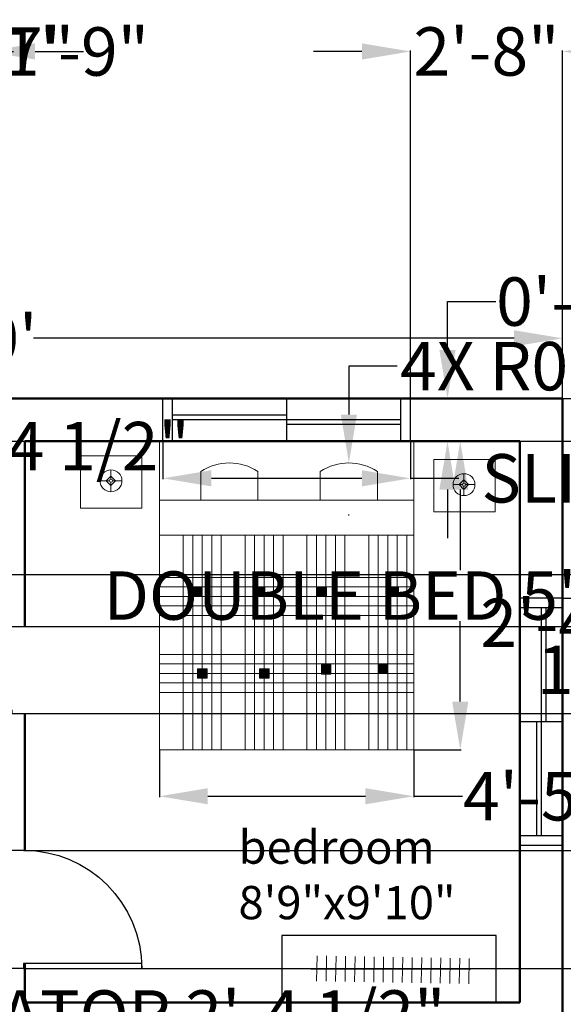
# Model space of a CAD drawing. Units: inches. Extents: x 19 to 1371, y 7 to 588.
# Tile 4 of 5: x 1092 to 1207, y 372 to 580. Entities that reach past the tile are written whole.
import ezdxf

# ---------------------------------------------------------------- set-up
doc = ezdxf.new("R2010")
doc.units = ezdxf.units.IN
doc.header["$MEASUREMENT"] = 0
for name, color, linetype, lineweight in [('A-ANNO-DIMS', 2, 'Continuous', 18), ('A-AREA-IDEN', 7, 'Continuous', 18), ('A-DOOR', 3, 'Continuous', 25), ('A-FLOR-CABN', 8, 'Continuous', 25), ('A-FURN', 8, 'Continuous', 18), ('A-FURN-PATT', 252, 'Continuous', 13), ('A-GLAZ', 4, 'Continuous', 25), ('A-WALL', 7, 'Continuous', 50)]:
    doc.layers.add(name, color=color, linetype=linetype, lineweight=lineweight)
doc.styles.get("Standard").update_dxf_attribs({"font": 'arial.ttf'})
doc.dimstyles.get("Standard").update_dxf_attribs({"dimtxt": 10.18, "dimasz": 10.18, "dimexe": 0.18, "dimexo": 0.0625, "dimgap": 0.09, "dimtad": 0, "dimtih": 1, "dimtoh": 1, "dimdec": 0, "dimzin": 0, "dimdsep": 46, "dimlunit": 3, "dimtxsty": 'Standard', "dimcen": 0.09, "dimadec": 0, "dimazin": 0, "dimtfac": 1, "dimtdec": 0, "dimtofl": 0, "dimtmove": 0, "dimatfit": 3, "dimfxl": 1, "dimtolj": 1, "dimtzin": 0, "dimarcsym": 0})

# ---------------------------------------------------------------- blocks, each defined once
blk = doc.blocks.new('*U2')
for p, q in [((0, 0), (0, -6)), ((40, 0), (40, -6))]:
    blk.add_line(p, q)
blk.add_lwpolyline([(0, 0), (0, 40), (1.75, 40), (1.75, 0)], close=True)
blk.add_arc((0, 0), 40, 0, 90)
blk = doc.blocks.new('Lamp - Table')
for p, q in [((0, 7), (0, 1)), ((-1, 0), (-7, 0)), ((0, 3), (-3, 0)), ((-3, 0), (0, -3)), ((3, 0), (0, 3)), ((0, -3), (3, 0)), ((1, 0), (7, 0)), ((0, -1), (0, -7))]:
    blk.add_line(p, q)
for radius in [7, 1]:
    blk.add_circle((0, 0), radius)
blk = doc.blocks.new('*D13')
at = {"layer": 'A-ANNO-DIMS', "color": 0, "lineweight": -2, "transparency": 16777216}
for p, q in [((966.44, 499.95), (966.44, 512.71)), ((976.62, 512.53), (1077.63, 512.53)), ((1196.26, 512.53), (1095.26, 512.53)), ((1206.44, 499.95), (1206.44, 512.71))]:
    blk.add_line(p, q, dxfattribs=at)
at = {"layer": 'A-ANNO-DIMS', "color": 0, "transparency": 16777216}
for points in [[(976.62, 514.22), (976.62, 510.83), (966.44, 512.53)], [(1196.26, 514.22), (1196.26, 510.83), (1206.44, 512.53)]]:
    blk.add_solid(points, dxfattribs=at)
at = {"layer": 'Defpoints', "color": 0, "transparency": 16777216}
for p in [(1206.44, 512.53), (966.44, 499.89), (1206.44, 499.89)]:
    blk.add_point(p, dxfattribs=at)
at = {"layer": 'A-ANNO-DIMS', "color": 0, "transparency": 16777216, "insert": (1086.44, 512.53), "char_height": 10.18, "attachment_point": 5}
blk.add_mtext("\\A1;20'", dxfattribs=at)
blk = doc.blocks.new('BED-DOUBLE-PLAN')
h = blk.add_hatch(color=256)
h.dxf.hatch_style = 1
h.paths.add_polyline_path([(9, 34.29), (7, 34.29), (7, 32.29), (9, 32.29)])
h = blk.add_hatch(color=256)
h.dxf.hatch_style = 1
h.paths.add_polyline_path([(22.14, 34.29), (20.14, 34.29), (20.14, 32.29), (22.14, 32.29)])
h = blk.add_hatch(color=256)
h.dxf.hatch_style = 1
h.paths.add_polyline_path([(35.09, 34.29), (33.09, 34.29), (33.09, 32.29), (35.09, 32.29)])
h = blk.add_hatch(color=256)
h.dxf.hatch_style = 1
h.paths.add_polyline_path([(50.26, 34.29), (48.26, 34.29), (48.26, 32.29), (50.26, 32.29)])
h = blk.add_hatch(color=256)
h.dxf.hatch_style = 1
h.paths.add_polyline_path([(10.04, 17.06), (8.04, 17.06), (8.04, 15.06), (10.04, 15.06)])
h = blk.add_hatch(color=256)
h.dxf.hatch_style = 1
h.paths.add_polyline_path([(23.04, 17.06), (21.04, 17.06), (21.04, 15.06), (23.04, 15.06)])
h = blk.add_hatch(color=256)
h.dxf.hatch_style = 1
h.paths.add_polyline_path([(36.04, 17.94), (34.04, 17.94), (34.04, 15.94), (36.04, 15.94)])
h = blk.add_hatch(color=256)
h.dxf.hatch_style = 1
h.paths.add_polyline_path([(47.99, 18.12), (45.99, 18.12), (45.99, 16.12), (47.99, 16.12)])
for p, q in [((8.7, 52.54), (8.7, 58.53)), ((20.7, 52.54), (20.7, 58.53)), ((33.82, 52.54), (33.82, 58.53)), ((45.82, 52.54), (45.82, 58.53)), ((53.49, 52.54), (0, 52.54)), ((0, 45.16), (53.49, 45.16)), ((0, 45.16), (5, 45.16)), ((5, 45.16), (5, 0)), ((7, 45.16), (7, 0)), ((9, 45.16), (9, 0)), ((11, 45.16), (11, 0)), ((13, 45.16), (13, 0)), ((18, 45.16), (18, 0)), ((20, 45.16), (20, 0)), ((22, 45.16), (22, 0)), ((24, 45.16), (24, 0)), ((26, 45.16), (26, 0)), ((31, 45.16), (31, 0)), ((33, 45.16), (33, 0)), ((35, 45.16), (35, 0)), ((37, 45.16), (37, 0)), ((39, 45.16), (39, 0)), ((44, 45.16), (44, 0)), ((46, 45.16), (46, 0)), ((48, 45.16), (48, 0)), ((50, 45.16), (50, 0)), ((52, 45.16), (52, 0)), ((0, 36.29), (53.49, 36.29)), ((0, 34.29), (53.49, 34.29)), ((0, 32.29), (53.49, 32.29)), ((0, 30.29), (53.49, 30.29)), ((0, 28.29), (53.49, 28.29)), ((0, 20.08), (53.49, 20.08)), ((0, 18.08), (53.49, 18.08)), ((0, 16.08), (53.49, 16.08)), ((0, 14.08), (53.49, 14.08)), ((0, 12.08), (53.49, 12.08)), ((5, 0), (5, 4.72)), ((5, 4.72), (5, 0))]:
    blk.add_line(p, q)
for points in [[(53.49, 64.91), (0, 64.91), (0, 0), (53.49, 0)], [(7, 34.29), (9, 34.29), (9, 32.29), (7, 32.29)], [(20.14, 34.29), (22.14, 34.29), (22.14, 32.29), (20.14, 32.29)], [(33.09, 34.29), (35.09, 34.29), (35.09, 32.29), (33.09, 32.29)], [(48.26, 34.29), (50.26, 34.29), (50.26, 32.29), (48.26, 32.29)], [(8.04, 17.06), (10.04, 17.06), (10.04, 15.06), (8.04, 15.06)], [(21.04, 17.06), (23.04, 17.06), (23.04, 15.06), (21.04, 15.06)], [(34.04, 17.94), (36.04, 17.94), (36.04, 15.94), (34.04, 15.94)], [(45.99, 18.12), (47.99, 18.12), (47.99, 16.12), (45.99, 16.12)]]:
    blk.add_lwpolyline(points, close=True)
for centre in [(14.7, 49.44), (39.82, 49.44)]:
    blk.add_arc(centre, 10.9, 56.5918, 123.4082)
blk = doc.blocks.new('WIN-SLIDING-48')
for p, q in [((0, 0), (0, 9)), ((2, 0), (2, 9)), ((26, 0), (26, 9)), ((50, 0), (50, 9)), ((52, 0), (52, 9)), ((26, 5.5), (2, 5.5)), ((50, 4.5), (2, 4.5)), ((50, 3.5), (26, 3.5))]:
    blk.add_line(p, q)
blk = doc.blocks.new('TABLE-BEDSIDE')
blk.add_lwpolyline([(0, 11.01), (12.94, 11.01), (12.94, 0), (0, 0)], close=True)
blk = doc.blocks.new('*D20')
at = {"layer": 'A-ANNO-DIMS', "color": 0, "lineweight": -2, "transparency": 16777216}
for p, q in [((1175.27, 490.89), (1185.12, 490.89)), ((1184.94, 480.71), (1184.94, 463.79)), ((1184.94, 436.16), (1184.94, 453.08)), ((1175.27, 425.98), (1185.12, 425.98))]:
    blk.add_line(p, q, dxfattribs=at)
at = {"layer": 'A-ANNO-DIMS', "color": 0, "transparency": 16777216}
for points in [[(1183.24, 480.71), (1186.64, 480.71), (1184.94, 490.89)], [(1183.24, 436.16), (1186.64, 436.16), (1184.94, 425.98)]]:
    blk.add_solid(points, dxfattribs=at)
at = {"layer": 'Defpoints', "color": 0, "transparency": 16777216}
for p in [(1175.2, 490.89), (1184.94, 490.89), (1175.2, 425.98)]:
    blk.add_point(p, dxfattribs=at)
at = {"layer": 'A-ANNO-DIMS', "color": 0, "transparency": 16777216, "insert": (1184.94, 458.44), "char_height": 10.18, "attachment_point": 5}
blk.add_mtext('\\A1;DOUBLE BED 5\'-5" TYP.', dxfattribs=at)
blk = doc.blocks.new('*D21')
at = {"layer": 'A-ANNO-DIMS', "color": 0, "lineweight": -2, "transparency": 16777216}
for p, q in [((1121.71, 425.92), (1121.71, 416.06)), ((1175.2, 425.92), (1175.2, 416.06)), ((1131.89, 416.24), (1165.02, 416.24)), ((1175.2, 416.24), (1185.38, 416.24))]:
    blk.add_line(p, q, dxfattribs=at)
at = {"layer": 'A-ANNO-DIMS', "color": 0, "transparency": 16777216}
for points in [[(1131.89, 417.94), (1131.89, 414.55), (1121.71, 416.24)], [(1165.02, 417.94), (1165.02, 414.55), (1175.2, 416.24)]]:
    blk.add_solid(points, dxfattribs=at)
at = {"layer": 'Defpoints', "color": 0, "transparency": 16777216}
for p in [(1121.71, 425.98), (1175.2, 425.98), (1175.2, 416.24)]:
    blk.add_point(p, dxfattribs=at)
at = {"layer": 'A-ANNO-DIMS', "color": 0, "transparency": 16777216, "insert": (1228.56, 416.24), "char_height": 10.18, "attachment_point": 5}
blk.add_mtext('\\A1;4\'-5 1/2" TYP.', dxfattribs=at)
blk = doc.blocks.new('*D30')
at = {"layer": 'A-ANNO-DIMS', "color": 0, "lineweight": -2, "transparency": 16777216}
for p, q in [((1122.46, 490.83), (1122.46, 482.91)), ((1174.46, 490.83), (1174.46, 482.91)), ((1132.64, 483.09), (1164.28, 483.09)), ((1174.46, 483.09), (1184.64, 483.09))]:
    blk.add_line(p, q, dxfattribs=at)
at = {"layer": 'A-ANNO-DIMS', "color": 0, "transparency": 16777216}
for points in [[(1132.64, 484.79), (1132.64, 481.39), (1122.46, 483.09)], [(1164.28, 484.79), (1164.28, 481.39), (1174.46, 483.09)]]:
    blk.add_solid(points, dxfattribs=at)
at = {"layer": 'Defpoints', "color": 0, "transparency": 16777216}
for p in [(1122.46, 490.89), (1174.46, 490.89), (1174.46, 483.09)]:
    blk.add_point(p, dxfattribs=at)
at = {"layer": 'A-ANNO-DIMS', "color": 0, "transparency": 16777216, "insert": (1279.33, 483.09), "char_height": 10.18, "attachment_point": 5}
blk.add_mtext('\\A1;SLIDING WINDOW 4\'-4" TYP.', dxfattribs=at)
blk = doc.blocks.new('*D31')
at = {"layer": 'A-ANNO-DIMS', "color": 0, "lineweight": -2, "transparency": 16777216}
for p, q in [((1182.26, 510.07), (1182.26, 520.25)), ((1182.26, 520.25), (1192.44, 520.25)), ((1174.52, 499.89), (1182.44, 499.89)), ((1174.52, 490.89), (1182.44, 490.89)), ((1182.26, 480.71), (1182.26, 470.53))]:
    blk.add_line(p, q, dxfattribs=at)
at = {"layer": 'A-ANNO-DIMS', "color": 0, "transparency": 16777216}
for points in [[(1180.56, 510.07), (1183.95, 510.07), (1182.26, 499.89)], [(1180.56, 480.71), (1183.95, 480.71), (1182.26, 490.89)]]:
    blk.add_solid(points, dxfattribs=at)
at = {"layer": 'Defpoints', "color": 0, "transparency": 16777216}
for p in [(1174.46, 499.89), (1182.26, 499.89), (1174.46, 490.89)]:
    blk.add_point(p, dxfattribs=at)
at = {"layer": 'A-ANNO-DIMS', "color": 0, "transparency": 16777216, "insert": (1223.55, 520.25), "char_height": 10.18, "attachment_point": 5}
blk.add_mtext('\\A1;0\'-9" TYP.', dxfattribs=at)
blk = doc.blocks.new('*D32')
at = {"layer": 'A-ANNO-DIMS', "color": 0, "lineweight": -2, "transparency": 16777216}
for p, q in [((992.39, 489.86), (982.21, 489.86)), ((1002.57, 487.44), (1002.57, 490.04)), ((1019.13, 487.44), (1019.13, 490.04)), ((1029.31, 489.86), (1039.49, 489.86))]:
    blk.add_line(p, q, dxfattribs=at)
at = {"layer": 'A-ANNO-DIMS', "color": 0, "transparency": 16777216}
for points in [[(992.39, 491.56), (992.39, 488.17), (1002.57, 489.86)], [(1029.31, 491.56), (1029.31, 488.17), (1019.13, 489.86)]]:
    blk.add_solid(points, dxfattribs=at)
at = {"layer": 'Defpoints', "color": 0, "transparency": 16777216}
for p in [(1019.13, 489.86), (1002.57, 487.38), (1019.13, 487.38)]:
    blk.add_point(p, dxfattribs=at)
at = {"layer": 'A-ANNO-DIMS', "color": 0, "transparency": 16777216, "insert": (1083.52, 489.86), "char_height": 10.18, "attachment_point": 5}
blk.add_mtext('\\A1;SINK 1\'-4 1/2"', dxfattribs=at)
blk = doc.blocks.new('*D36')
at = {"layer": 'A-ANNO-DIMS', "color": 0, "lineweight": -2, "transparency": 16777216}
for p, q in [((980.44, 374.59), (980.44, 370.17)), ((1009.08, 374.59), (1009.08, 370.17)), ((990.62, 370.35), (998.9, 370.35)), ((1009.08, 370.35), (1019.26, 370.35))]:
    blk.add_line(p, q, dxfattribs=at)
at = {"layer": 'A-ANNO-DIMS', "color": 0, "transparency": 16777216}
for points in [[(990.62, 372.05), (990.62, 368.66), (980.44, 370.35)], [(998.9, 372.05), (998.9, 368.66), (1009.08, 370.35)]]:
    blk.add_solid(points, dxfattribs=at)
at = {"layer": 'Defpoints', "color": 0, "transparency": 16777216}
for p in [(980.44, 374.65), (1009.08, 374.65), (1009.08, 370.35)]:
    blk.add_point(p, dxfattribs=at)
at = {"layer": 'A-ANNO-DIMS', "color": 0, "transparency": 16777216, "insert": (1102.94, 370.35), "char_height": 10.18, "attachment_point": 5}
blk.add_mtext('\\A1;REFRIGERATOR 2\'-4 1/2"', dxfattribs=at)
blk = doc.blocks.new('*D46')
at = {"layer": 'A-ANNO-DIMS', "color": 0, "lineweight": -2, "transparency": 16777216}
for p, q in [((1035.21, 572.84), (1025.03, 572.84)), ((1045.39, 211.95), (1045.39, 573.02)), ((1085.39, 211.95), (1085.39, 573.02)), ((1095.57, 572.84), (1105.75, 572.84))]:
    blk.add_line(p, q, dxfattribs=at)
at = {"layer": 'A-ANNO-DIMS', "color": 0, "transparency": 16777216}
for points in [[(1035.21, 574.54), (1035.21, 571.14), (1045.39, 572.84)], [(1095.57, 574.54), (1095.57, 571.14), (1085.39, 572.84)]]:
    blk.add_solid(points, dxfattribs=at)
at = {"layer": 'Defpoints', "color": 0, "transparency": 16777216}
for p in [(1085.39, 572.84), (1045.39, 211.89), (1085.39, 211.89)]:
    blk.add_point(p, dxfattribs=at)
at = {"layer": 'A-ANNO-DIMS', "color": 0, "transparency": 16777216, "insert": (1065.39, 572.84), "char_height": 10.18, "attachment_point": 5}
blk.add_mtext('\\A1;3\'-4"', dxfattribs=at)
blk = doc.blocks.new('*D48')
at = {"layer": 'A-ANNO-DIMS', "color": 0, "lineweight": -2, "transparency": 16777216}
for p, q in [((1228.39, 404.87), (1228.39, 415.05)), ((1228.39, 415.05), (1238.57, 415.05)), ((1093.5, 404.87), (1228.57, 404.87)), ((1228.39, 390.2), (1228.39, 394.69)), ((1093.23, 380.02), (1228.57, 380.02))]:
    blk.add_line(p, q, dxfattribs=at)
at = {"layer": 'A-ANNO-DIMS', "color": 0, "transparency": 16777216}
for points in [[(1226.7, 394.69), (1230.09, 394.69), (1228.39, 404.87)], [(1226.7, 390.2), (1230.09, 390.2), (1228.39, 380.02)]]:
    blk.add_solid(points, dxfattribs=at)
at = {"layer": 'Defpoints', "color": 0, "transparency": 16777216}
for p in [(1093.44, 404.87), (1228.39, 404.87), (1093.17, 380.02)]:
    blk.add_point(p, dxfattribs=at)
at = {"layer": 'A-ANNO-DIMS', "color": 0, "transparency": 16777216, "insert": (1252.28, 415.05), "char_height": 10.18, "attachment_point": 5}
blk.add_mtext('\\A1;2\'-1"', dxfattribs=at)
blk = doc.blocks.new('*D50')
at = {"layer": 'A-ANNO-DIMS', "color": 0, "lineweight": -2, "transparency": 16777216}
for p, q in [((1228.39, 462.14), (1228.39, 472.32)), ((1093.5, 451.96), (1228.57, 451.96)), ((1093.5, 433.64), (1228.57, 433.64)), ((1228.39, 423.46), (1228.39, 413.28))]:
    blk.add_line(p, q, dxfattribs=at)
at = {"layer": 'A-ANNO-DIMS', "color": 0, "transparency": 16777216}
for points in [[(1226.7, 462.14), (1230.09, 462.14), (1228.39, 451.96)], [(1226.7, 423.46), (1230.09, 423.46), (1228.39, 433.64)]]:
    blk.add_solid(points, dxfattribs=at)
at = {"layer": 'Defpoints', "color": 0, "transparency": 16777216}
for p in [(1093.44, 451.96), (1228.39, 451.96), (1093.44, 433.64)]:
    blk.add_point(p, dxfattribs=at)
at = {"layer": 'A-ANNO-DIMS', "color": 0, "transparency": 16777216, "insert": (1228.39, 442.8), "char_height": 10.18, "attachment_point": 5}
blk.add_mtext('\\A1;1\'-6 1/2"', dxfattribs=at)
blk = doc.blocks.new('*D61')
at = {"layer": 'A-ANNO-DIMS', "color": 0, "lineweight": -2, "transparency": 16777216}
for p, q in [((1206.5, 499.89), (1228.57, 499.89)), ((1228.39, 489.71), (1228.39, 484.18)), ((1228.39, 468.07), (1228.39, 473.6)), ((1206.5, 457.89), (1228.57, 457.89))]:
    blk.add_line(p, q, dxfattribs=at)
at = {"layer": 'A-ANNO-DIMS', "color": 0, "transparency": 16777216}
for points in [[(1226.7, 489.71), (1230.09, 489.71), (1228.39, 499.89)], [(1226.7, 468.07), (1230.09, 468.07), (1228.39, 457.89)]]:
    blk.add_solid(points, dxfattribs=at)
at = {"layer": 'Defpoints', "color": 0, "transparency": 16777216}
for p in [(1206.44, 499.89), (1206.44, 457.89), (1228.39, 457.89)]:
    blk.add_point(p, dxfattribs=at)
at = {"layer": 'A-ANNO-DIMS', "color": 0, "transparency": 16777216, "insert": (1228.39, 478.89), "char_height": 10.18, "attachment_point": 5}
blk.add_mtext('\\A1;3\'-6"', dxfattribs=at)
blk = doc.blocks.new('*D62')
at = {"layer": 'A-ANNO-DIMS', "color": 0, "lineweight": -2, "transparency": 16777216}
for p, q in [((1228.39, 377.07), (1228.39, 387.25)), ((1197.5, 366.89), (1228.57, 366.89)), ((1197.5, 359.89), (1228.57, 359.89)), ((1228.39, 349.71), (1228.39, 339.53)), ((1228.39, 339.53), (1218.21, 339.53))]:
    blk.add_line(p, q, dxfattribs=at)
at = {"layer": 'A-ANNO-DIMS', "color": 0, "transparency": 16777216}
for points in [[(1226.7, 377.07), (1230.09, 377.07), (1228.39, 366.89)], [(1226.7, 349.71), (1230.09, 349.71), (1228.39, 359.89)]]:
    blk.add_solid(points, dxfattribs=at)
at = {"layer": 'Defpoints', "color": 0, "transparency": 16777216}
for p in [(1197.44, 366.89), (1197.44, 359.89), (1228.39, 359.89)]:
    blk.add_point(p, dxfattribs=at)
at = {"layer": 'A-ANNO-DIMS', "color": 0, "transparency": 16777216, "insert": (1204.59, 339.53), "char_height": 10.18, "attachment_point": 5}
blk.add_mtext('\\A1;0\'-7"', dxfattribs=at)
blk = doc.blocks.new('*D64')
at = {"layer": 'A-ANNO-DIMS', "color": 0, "lineweight": -2, "transparency": 16777216}
for p, q in [((1037.26, 572.84), (1027.08, 572.84)), ((1047.44, 490.95), (1047.44, 573.02)), ((1054.44, 490.95), (1054.44, 573.02)), ((1064.62, 572.84), (1074.8, 572.84))]:
    blk.add_line(p, q, dxfattribs=at)
at = {"layer": 'A-ANNO-DIMS', "color": 0, "transparency": 16777216}
for points in [[(1037.26, 574.54), (1037.26, 571.14), (1047.44, 572.84)], [(1064.62, 574.54), (1064.62, 571.14), (1054.44, 572.84)]]:
    blk.add_solid(points, dxfattribs=at)
at = {"layer": 'Defpoints', "color": 0, "transparency": 16777216}
for p in [(1054.44, 572.84), (1047.44, 490.89), (1054.44, 490.89)]:
    blk.add_point(p, dxfattribs=at)
at = {"layer": 'A-ANNO-DIMS', "color": 0, "transparency": 16777216, "insert": (1088.42, 572.84), "char_height": 10.18, "attachment_point": 5}
blk.add_mtext('\\A1;0\'-7"', dxfattribs=at)
blk = doc.blocks.new('*D65')
at = {"layer": 'A-ANNO-DIMS', "color": 0, "lineweight": -2, "transparency": 16777216}
for p, q in [((1164.28, 572.84), (1154.1, 572.84)), ((1174.46, 499.95), (1174.46, 573.02)), ((1206.44, 499.95), (1206.44, 573.02)), ((1216.62, 572.84), (1226.8, 572.84))]:
    blk.add_line(p, q, dxfattribs=at)
at = {"layer": 'A-ANNO-DIMS', "color": 0, "transparency": 16777216}
for points in [[(1164.28, 574.54), (1164.28, 571.14), (1174.46, 572.84)], [(1216.62, 574.54), (1216.62, 571.14), (1206.44, 572.84)]]:
    blk.add_solid(points, dxfattribs=at)
at = {"layer": 'Defpoints', "color": 0, "transparency": 16777216}
for p in [(1206.44, 572.84), (1174.46, 499.89), (1206.44, 499.89)]:
    blk.add_point(p, dxfattribs=at)
at = {"layer": 'A-ANNO-DIMS', "color": 0, "transparency": 16777216, "insert": (1190.45, 572.84), "char_height": 10.18, "attachment_point": 5}
blk.add_mtext('\\A1;2\'-8"', dxfattribs=at)
blk = doc.blocks.new('*D68')
at = {"layer": 'A-ANNO-DIMS', "color": 0, "lineweight": -2, "transparency": 16777216}
for p, q in [((1059.87, 490.95), (1059.87, 573.02)), ((1070.05, 572.84), (1070.69, 572.84)), ((1080.87, 490.95), (1080.87, 573.02)), ((1080.87, 572.84), (1091.05, 572.84))]:
    blk.add_line(p, q, dxfattribs=at)
at = {"layer": 'A-ANNO-DIMS', "color": 0, "transparency": 16777216}
for points in [[(1070.05, 574.54), (1070.05, 571.14), (1059.87, 572.84)], [(1070.69, 574.54), (1070.69, 571.14), (1080.87, 572.84)]]:
    blk.add_solid(points, dxfattribs=at)
at = {"layer": 'Defpoints', "color": 0, "transparency": 16777216}
for p in [(1080.87, 572.84), (1059.87, 490.89), (1080.87, 490.89)]:
    blk.add_point(p, dxfattribs=at)
at = {"layer": 'A-ANNO-DIMS', "color": 0, "transparency": 16777216, "insert": (1104.19, 572.84), "char_height": 10.18, "attachment_point": 5}
blk.add_mtext('\\A1;1\'-9"', dxfattribs=at)
blk = doc.blocks.new('*D69')
at = {"layer": 'A-ANNO-DIMS', "color": 0, "lineweight": -2, "transparency": 16777216}
for p, q in [((1080.93, 490.89), (1228.57, 490.89)), ((1228.39, 480.71), (1228.39, 473.07)), ((1070.43, 462.89), (1228.57, 462.89)), ((1228.39, 462.89), (1228.39, 452.71)), ((1228.39, 452.71), (1218.21, 452.71))]:
    blk.add_line(p, q, dxfattribs=at)
at = {"layer": 'A-ANNO-DIMS', "color": 0, "transparency": 16777216}
for points in [[(1226.7, 480.71), (1230.09, 480.71), (1228.39, 490.89)], [(1226.7, 473.07), (1230.09, 473.07), (1228.39, 462.89)]]:
    blk.add_solid(points, dxfattribs=at)
at = {"layer": 'Defpoints', "color": 0, "transparency": 16777216}
for p in [(1080.87, 490.89), (1070.37, 462.89), (1228.39, 462.89)]:
    blk.add_point(p, dxfattribs=at)
at = {"layer": 'A-ANNO-DIMS', "color": 0, "transparency": 16777216, "insert": (1204.51, 452.71), "char_height": 10.18, "attachment_point": 5}
blk.add_mtext('\\A1;2\'-4"', dxfattribs=at)
blk = doc.blocks.new('*D75')
at = {"layer": 'A-ANNO-DIMS', "color": 0, "lineweight": -2, "transparency": 16777216}
for p, q in [((1171.71, 506.67), (1161.53, 506.67)), ((1161.53, 506.67), (1161.53, 496.49)), ((1161.44, 475.42), (1161.62, 475.42)), ((1161.53, 475.33), (1161.53, 475.51))]:
    blk.add_line(p, q, dxfattribs=at)
at = {"layer": 'A-ANNO-DIMS', "color": 0, "transparency": 16777216}
blk.add_solid([(1159.84, 496.49), (1163.23, 496.49), (1161.53, 486.31)], dxfattribs=at)
at = {"layer": 'Defpoints', "color": 0, "transparency": 16777216}
for p in [(1161.53, 486.31), (1161.53, 475.42)]:
    blk.add_point(p, dxfattribs=at)
at = {"layer": 'A-ANNO-DIMS', "color": 0, "transparency": 16777216, "insert": (1205.3, 506.67), "char_height": 10.18, "attachment_point": 5}
blk.add_mtext('\\A1;4X R0\'-11"', dxfattribs=at)

msp = doc.modelspace()

# ---------------------------------------------------------------- hatches: boundary and pattern name
at = {"layer": 'A-FURN-PATT'}
h = msp.add_hatch(dxfattribs=at)
h.set_pattern_fill('ANSI31', color=256, scale=15.99746, angle=43.9757, style=0)
h.paths.add_polyline_path([(1154.7, 377.38), (1186.79, 376.81), (1186.89, 382.15), (1154.79, 382.72)])

# ---------------------------------------------------------------- linework, layer by layer
at = {"layer": 'A-FLOR-CABN'}
for p, q in [((1192.51, 386.93), (1147.46, 386.93)), ((1147.46, 386.93), (1147.46, 372.89)), ((1192.51, 372.89), (1192.51, 386.93)), ((1153.52, 379.99), (1187.16, 379.99))]:
    msp.add_line(p, q, dxfattribs=at)
at = {"layer": 'A-WALL'}
for p, q in [((966.44, 499.89), (1206.44, 499.89)), ((1206.44, 499.89), (1206.44, 139.89)), ((1093.44, 490.89), (1197.44, 490.89)), ((1093.44, 451.96), (1093.44, 490.89)), ((1197.44, 490.89), (1197.44, 372.89)), ((1093.44, 404.87), (1093.44, 433.64)), ((1093.44, 372.89), (1093.44, 381.11)), ((1093.44, 372.89), (1197.44, 372.89))]:
    msp.add_line(p, q, dxfattribs=at)

# ---------------------------------------------------------------- block references
at = {"layer": 'A-DOOR'}
for p, xscale, yscale, zscale, rotation in [((1090.69, 433.64), 0.4579245056729436, 0.4579245056729436, 0.4579245056729436, 90), ((1093.17, 380.02), -0.6212879094378088, 0.6212879094378088, 0.6212879094378088, 270)]:
    msp.add_blockref('*U2', p, dxfattribs=dict(at, xscale=xscale, yscale=yscale, zscale=zscale, rotation=rotation))
at = {"layer": 'A-FURN'}
for name, p in [('BED-DOUBLE-PLAN', (1121.71, 425.98)), ('TABLE-BEDSIDE', (1105.11, 476.84)), ('TABLE-BEDSIDE', (1179.36, 476.05))]:
    msp.add_blockref(name, p, dxfattribs=at)
at = {"layer": 'A-FURN', "xscale": 0.3285708312946518, "yscale": 0.3285708312946518, "zscale": 0.3285708312946518}
for p in [(1111.53, 482.58), (1185.72, 481.76)]:
    msp.add_blockref('Lamp - Table', p, dxfattribs=at)
at = {"layer": 'A-GLAZ'}
msp.add_blockref('WIN-SLIDING-48', (1122.46, 490.89), dxfattribs=at)
at = {"layer": 'A-GLAZ', "rotation": 90.00000000000011}
msp.add_blockref('WIN-SLIDING-48', (1206.44, 405.89), dxfattribs=at)

# ---------------------------------------------------------------- texts
at = {"layer": 'A-AREA-IDEN', "insert": (1138.33, 409.05), "char_height": 7, "attachment_point": 1}
msp.add_mtext_dynamic_manual_height_columns('bedroom\\P8\'9"x9\'10"', width=53.7683, gutter_width=1, heights=[0], dxfattribs=at)

# ---------------------------------------------------------------- dimensions: what is measured, and where the dimension line sits
at = {"layer": 'A-ANNO-DIMS'}
for base, p1, p2, override, picture, middle in [((1085.39, 572.84), (1045.39, 211.89), (1085.39, 211.89), {"dimdec": 1, "dimlfac": 1, "dimrnd": 0, "dimzin": 1, "dimdsep": 46, "dimlunit": 4, "dimfrac": 2}, '*D46', (1065.39, 572.84)), ((1054.44, 572.84), (1047.44, 490.89), (1054.44, 490.89), {"dimdec": 1, "dimlfac": 1, "dimrnd": 0, "dimzin": 1, "dimdsep": 46, "dimlunit": 4, "dimfrac": 2}, '*D64', (1088.42, 572.84)), ((1080.87, 572.84), (1059.87, 490.89), (1080.87, 490.89), {"dimdec": 1, "dimlfac": 1, "dimrnd": 0, "dimzin": 1, "dimdsep": 46, "dimlunit": 4, "dimfrac": 2}, '*D68', (1104.19, 572.84)), ((1206.44, 572.84), (1174.46, 499.89), (1206.44, 499.89), {"dimdec": 1, "dimlfac": 1, "dimrnd": 0, "dimzin": 1, "dimdsep": 46, "dimlunit": 4, "dimfrac": 2}, '*D65', (1190.45, 572.84)), ((1206.44, 512.53), (966.44, 499.89), (1206.44, 499.89), {"dimclrd": 0, "dimclre": 0, "dimclrt": 0}, '*D13', (1086.44, 512.53))]:
    dim = msp.add_linear_dim(base=base, p1=p1, p2=p2, dimstyle='Standard', override=override, dxfattribs=at)
    dim.commit()
    dim.dimension.update_dxf_attribs({"geometry": picture, "text_midpoint": middle})
for base, p1, p2, text, picture, middle in [((1182.26, 499.89), (1174.46, 490.89), (1174.46, 499.89), '<> TYP.', '*D31', (1223.55, 520.25)), ((1184.94, 490.89), (1175.2, 425.98), (1175.2, 490.89), 'DOUBLE BED <> TYP.', '*D20', (1184.94, 458.44))]:
    dim = msp.add_linear_dim(base=base, p1=p1, p2=p2, angle=90, text=text, dimstyle='Standard', override={"dimdec": 1, "dimlfac": 1, "dimrnd": 0, "dimzin": 1, "dimdsep": 46, "dimlunit": 4, "dimfrac": 2}, dxfattribs=at)
    dim.commit()
    dim.dimension.update_dxf_attribs({"geometry": picture, "text_midpoint": middle})
dim = msp.add_radius_dim(center=(1161.53, 475.42), mpoint=(1161.53, 486.31), text='4X <>', dimstyle='Standard', override={"dimdec": 1, "dimlfac": 1, "dimrnd": 0, "dimzin": 1, "dimdsep": 46, "dimlunit": 4, "dimfrac": 2}, dxfattribs=at)
dim.commit()
dim.dimension.update_dxf_attribs({"geometry": '*D75', "text_midpoint": (1205.3, 506.67)})
for base, p1, p2, text, picture, middle in [((1019.13, 489.86), (1002.57, 487.38), (1019.13, 487.38), 'SINK <>', '*D32', (1083.52, 489.86)), ((1174.46, 483.09), (1122.46, 490.89), (1174.46, 490.89), 'SLIDING WINDOW <> TYP.', '*D30', (1279.33, 483.09)), ((1175.2, 416.24), (1121.71, 425.98), (1175.2, 425.98), '<> TYP.', '*D21', (1228.56, 416.24)), ((1009.08, 370.35), (980.44, 374.65), (1009.08, 374.65), 'REFRIGERATOR <>', '*D36', (1102.94, 370.35))]:
    dim = msp.add_linear_dim(base=base, p1=p1, p2=p2, text=text, dimstyle='Standard', override={"dimdec": 1, "dimlfac": 1, "dimrnd": 0, "dimzin": 1, "dimdsep": 46, "dimlunit": 4, "dimfrac": 2}, dxfattribs=at)
    dim.commit()
    dim.dimension.update_dxf_attribs({"geometry": picture, "text_midpoint": middle})
for base, p1, p2, picture, middle in [((1228.39, 457.89), (1206.44, 499.89), (1206.44, 457.89), '*D61', (1228.39, 478.89)), ((1228.39, 462.89), (1080.87, 490.89), (1070.37, 462.89), '*D69', (1204.51, 452.71)), ((1228.39, 451.96), (1093.44, 433.64), (1093.44, 451.96), '*D50', (1228.39, 442.8)), ((1228.39246, 404.87298), (1093.17018, 380.02295), (1093.44246, 404.87298), '*D48', (1252.27977, 415.05298)), ((1228.39, 359.89), (1197.44, 366.89), (1197.44, 359.89), '*D62', (1204.59, 339.53))]:
    dim = msp.add_linear_dim(base=base, p1=p1, p2=p2, angle=90, dimstyle='Standard', override={"dimdec": 1, "dimlfac": 1, "dimrnd": 0, "dimzin": 1, "dimdsep": 46, "dimlunit": 4, "dimfrac": 2}, dxfattribs=at)
    dim.commit()
    dim.dimension.update_dxf_attribs({"geometry": picture, "text_midpoint": middle})

doc.saveas('drawing.dxf')
